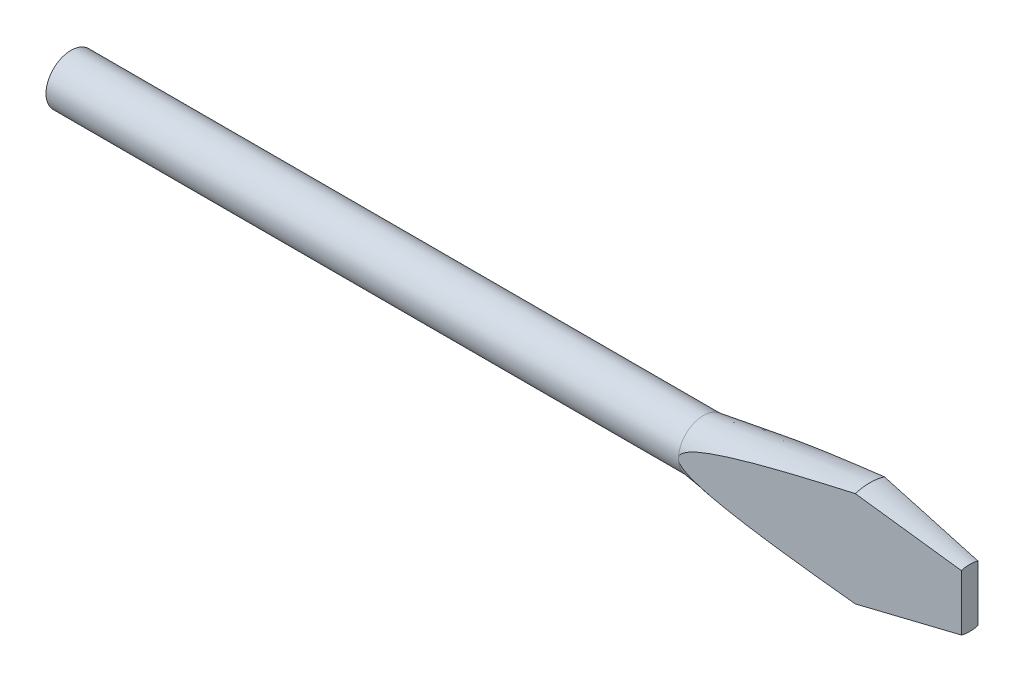
ISO-10303-21;
HEADER;
FILE_DESCRIPTION(('STEP AP214'),'2;1');
FILE_NAME('part.step','',(''),(''),'','','');
FILE_SCHEMA(('AUTOMOTIVE_DESIGN { 1 0 10303 214 1 1 1 1 }'));
ENDSEC;
DATA;
#1=APPLICATION_CONTEXT('core data for automotive mechanical design processes');
#2=APPLICATION_PROTOCOL_DEFINITION('international standard','automotive_design',2000,#1);
#3=PRODUCT_CONTEXT('',#1,'mechanical');
#4=PRODUCT('Part','Part','',(#3));
#5=PRODUCT_RELATED_PRODUCT_CATEGORY('part','',(#4));
#6=PRODUCT_DEFINITION_FORMATION('','',#4);
#7=PRODUCT_DEFINITION_CONTEXT('part definition',#1,'design');
#8=PRODUCT_DEFINITION('design','',#6,#7);
#9=PRODUCT_DEFINITION_SHAPE('','',#8);
#10=(LENGTH_UNIT() NAMED_UNIT(*) SI_UNIT(.MILLI.,.METRE.));
#11=(NAMED_UNIT(*) PLANE_ANGLE_UNIT() SI_UNIT($,.RADIAN.));
#12=(NAMED_UNIT(*) SI_UNIT($,.STERADIAN.) SOLID_ANGLE_UNIT());
#13=UNCERTAINTY_MEASURE_WITH_UNIT(LENGTH_MEASURE(1.E-05),#10,'distance_accuracy_value','');
#14=(GEOMETRIC_REPRESENTATION_CONTEXT(3) GLOBAL_UNCERTAINTY_ASSIGNED_CONTEXT((#13)) GLOBAL_UNIT_ASSIGNED_CONTEXT((#10,
#11,#12)) REPRESENTATION_CONTEXT('',''));
#15=CARTESIAN_POINT('',(0.,0.,0.));
#16=DIRECTION('',(0.,0.,1.));
#17=DIRECTION('',(1.,0.,0.));
#18=AXIS2_PLACEMENT_3D('',#15,#16,#17);
#19=CARTESIAN_POINT('',(96.,0.,0.));
#20=DIRECTION('',(1.,0.,0.));
#21=DIRECTION('',(0.,0.,-1.));
#22=AXIS2_PLACEMENT_3D('',#19,#20,#21);
#23=CONICAL_SURFACE('',#22,6.00000000000001,0.148889947609498);
#24=CARTESIAN_POINT('',(96.0002,5.73915531683399,1.7499875));
#25=CARTESIAN_POINT('',(95.5726499864452,5.66395600184694,1.77670937584718));
#26=CARTESIAN_POINT('',(95.1451987285646,5.58819220301967,1.80342507946472));
#27=CARTESIAN_POINT('',(94.2905240343786,5.43537319976455,1.85684224785134));
#28=CARTESIAN_POINT('',(93.8633005992586,5.35831798868393,1.88354371254634));
#29=CARTESIAN_POINT('',(92.5819083567461,5.12495166818705,1.96363072770337));
#30=CARTESIAN_POINT('',(91.7281335000303,4.96646016337192,2.01699165624811));
#31=CARTESIAN_POINT('',(90.019979848679,4.64146537301027,2.12375125945756));
#32=CARTESIAN_POINT('',(89.1656044854042,4.47494384895681,2.17714971966224));
#33=CARTESIAN_POINT('',(87.8856595668706,4.21721361058394,2.25714627707059));
#34=CARTESIAN_POINT('',(87.4592926054404,4.12998137074823,2.28379421215998));
#35=CARTESIAN_POINT('',(86.6072250559407,3.95231391396148,2.33704843400371));
#36=CARTESIAN_POINT('',(86.1815244633616,3.86187871878447,2.3636547210399));
#37=CARTESIAN_POINT('',(85.3312138352515,3.67715280873303,2.41679913529678));
#38=CARTESIAN_POINT('',(84.9066033099843,3.58286436326236,2.44333729312598));
#39=CARTESIAN_POINT('',(84.0584687809175,3.38939992425362,2.49634570119266));
#40=CARTESIAN_POINT('',(83.6349448230058,3.29022372775725,2.52281594856214));
#41=CARTESIAN_POINT('',(82.7896523378295,3.0856296102126,2.57564672888565));
#42=CARTESIAN_POINT('',(82.3678829429874,2.98021530209393,2.60200731606329));
#43=CARTESIAN_POINT('',(81.5265366338004,2.7609833456918,2.65459146038747));
#44=CARTESIAN_POINT('',(81.1069595251366,2.6471664562026,2.68081502967896));
#45=CARTESIAN_POINT('',(80.4071377845036,2.44647984326731,2.72455388846852));
#46=CARTESIAN_POINT('',(80.1259604528363,2.3628856653321,2.74212747169773));
#47=CARTESIAN_POINT('',(79.5658035182563,2.18838498181537,2.77713728010898));
#48=CARTESIAN_POINT('',(79.2868241923529,2.09747757025181,2.79457348797794));
#49=CARTESIAN_POINT('',(78.8218721534036,1.93636200836302,2.82363299041227));
#50=CARTESIAN_POINT('',(78.6349406666478,1.86894212685137,2.83531620833451));
#51=CARTESIAN_POINT('',(78.2634966175948,1.7278851236311,2.85853146140032));
#52=CARTESIAN_POINT('',(78.0789829462789,1.65425097650611,2.87006356585756));
#53=CARTESIAN_POINT('',(77.7692838551867,1.52206073077131,2.88941975905083));
#54=CARTESIAN_POINT('',(77.6431521485968,1.46574692133821,2.89730299071269));
#55=CARTESIAN_POINT('',(77.3933332707296,1.34752106226873,2.9129166705794));
#56=CARTESIAN_POINT('',(77.2696490920777,1.2856026199415,2.92064693174514));
#57=CARTESIAN_POINT('',(77.0267142840414,1.15443353979788,2.93583035724741));
#58=CARTESIAN_POINT('',(76.9074482122798,1.08521251318701,2.94328448673251));
#59=CARTESIAN_POINT('',(76.7339240635911,0.973178626859508,2.95412974602555));
#60=CARTESIAN_POINT('',(76.6770192579268,0.934499081121033,2.95768629637957));
#61=CARTESIAN_POINT('',(76.5657102745783,0.853705624728018,2.96464310783886));
#62=CARTESIAN_POINT('',(76.5113045369663,0.811593903283039,2.9680434664396));
#63=CARTESIAN_POINT('',(76.4109105801654,0.72706727244706,2.97431808873966));
#64=CARTESIAN_POINT('',(76.3646075046718,0.685031882048725,2.97721203095801));
#65=CARTESIAN_POINT('',(76.2763771477047,0.596432252281046,2.98272642826845));
#66=CARTESIAN_POINT('',(76.2344516319525,0.549866199953424,2.98534677300297));
#67=CARTESIAN_POINT('',(76.1638427175753,0.45942401347692,2.98975983015154));
#68=CARTESIAN_POINT('',(76.1341161979311,0.416380117894299,2.9916177376293));
#69=CARTESIAN_POINT('',(76.0817558589671,0.326142818282468,2.99489025881455));
#70=CARTESIAN_POINT('',(76.0591029434721,0.278961034526327,2.99630606603299));
#71=CARTESIAN_POINT('',(76.0287140728707,0.194604229642632,2.99820537044558));
#72=CARTESIAN_POINT('',(76.0185798334005,0.158308409565959,2.99883876041247));
#73=CARTESIAN_POINT('',(76.0045422133693,0.0845314040429726,2.99971611166441));
#74=CARTESIAN_POINT('',(76.0006312023623,0.0470517277746489,2.99996054985235));
#75=CARTESIAN_POINT('',(75.9995096958247,-0.0280966250484533,3.00003064401095));
#76=CARTESIAN_POINT('',(76.0023143668073,-0.0657655373225097,2.99985535207454));
#77=CARTESIAN_POINT('',(76.0142997316137,-0.140076870201679,2.99910626677414));
#78=CARTESIAN_POINT('',(76.0234878180765,-0.176718049349556,2.99853201137021));
#79=CARTESIAN_POINT('',(76.0511279458859,-0.259755019962619,2.99680450338213));
#80=CARTESIAN_POINT('',(76.0716181053519,-0.305460096964524,2.9955238684155));
#81=CARTESIAN_POINT('',(76.1194671645362,-0.393071508670082,2.99253330221648));
#82=CARTESIAN_POINT('',(76.1468420011463,-0.434968718132925,2.99082237492835));
#83=CARTESIAN_POINT('',(76.2308440864035,-0.548326904047211,2.98557224459977));
#84=CARTESIAN_POINT('',(76.2929683259939,-0.615651134591144,2.98168947962538));
#85=CARTESIAN_POINT('',(76.3922617223705,-0.709891572697012,2.97548364235184));
#86=CARTESIAN_POINT('',(76.4264549871577,-0.740236849569235,2.97334656330264));
#87=CARTESIAN_POINT('',(76.4964507424118,-0.79899898280661,2.96897182859926));
#88=CARTESIAN_POINT('',(76.5322524275458,-0.827416786752987,2.96673422327838));
#89=CARTESIAN_POINT('',(76.6465227232719,-0.91404425240467,2.9595923297955));
#90=CARTESIAN_POINT('',(76.7271721633252,-0.969346316998965,2.95455173979217));
#91=CARTESIAN_POINT('',(76.8919404364799,-1.07454240034944,2.94425372272));
#92=CARTESIAN_POINT('',(76.976062560228,-1.12443111923898,2.93899608998575));
#93=CARTESIAN_POINT('',(77.1468690560182,-1.2201956458567,2.92832068399886));
#94=CARTESIAN_POINT('',(77.2335603878113,-1.26605890270873,2.92290247576179));
#95=CARTESIAN_POINT('',(77.408604494444,-1.3544990689602,2.91196221909725));
#96=CARTESIAN_POINT('',(77.4969576273404,-1.39707525979243,2.90644014829122));
#97=CARTESIAN_POINT('',(77.7652954457971,-1.52153396282849,2.88966903463768));
#98=CARTESIAN_POINT('',(77.9471427155521,-1.59938497219916,2.87830358027799));
#99=CARTESIAN_POINT('',(78.2219023740701,-1.71052769479077,2.86113110162061));
#100=CARTESIAN_POINT('',(78.3137282495272,-1.74660327765731,2.85539198440454));
#101=CARTESIAN_POINT('',(78.4979891948311,-1.81715507612519,2.84387567532305));
#102=CARTESIAN_POINT('',(78.5904242395672,-1.85163135718625,2.83809848502705));
#103=CARTESIAN_POINT('',(78.8650697321673,-1.95176495296288,2.82093314173954));
#104=CARTESIAN_POINT('',(79.0479889859014,-2.01546798574804,2.80950068838116));
#105=CARTESIAN_POINT('',(79.4152004881255,-2.13878844706536,2.78654996949216));
#106=CARTESIAN_POINT('',(79.5994928565958,-2.19840551381847,2.77503169646276));
#107=CARTESIAN_POINT('',(79.9691529686513,-2.31437396895296,2.75192793945929));
#108=CARTESIAN_POINT('',(80.1545210055809,-2.37072441554196,2.74034243715119));
#109=CARTESIAN_POINT('',(80.5260554835113,-2.48072422260111,2.71712153228054));
#110=CARTESIAN_POINT('',(80.7122219450877,-2.53437351300235,2.70548612843202));
#111=CARTESIAN_POINT('',(81.2723101398846,-2.69213137866171,2.67048061625721));
#112=CARTESIAN_POINT('',(81.6471820551321,-2.79285333142643,2.64705112155424));
#113=CARTESIAN_POINT('',(82.3985506606079,-2.98767999779727,2.600090583712));
#114=CARTESIAN_POINT('',(82.7750470750032,-3.08178579123681,2.5765595578123));
#115=CARTESIAN_POINT('',(83.5271214588481,-3.26438779545831,2.52955490882199));
#116=CARTESIAN_POINT('',(83.9026924696457,-3.35291287140362,2.50608172064714));
#117=CARTESIAN_POINT('',(84.6547626031726,-3.52596598586649,2.45907733730171));
#118=CARTESIAN_POINT('',(85.0312617621282,-3.6104938656868,2.43554613986699));
#119=CARTESIAN_POINT('',(85.7846632666543,-3.77621867302195,2.3884585458341));
#120=CARTESIAN_POINT('',(86.1615650257566,-3.85741828350884,2.36490218589021));
#121=CARTESIAN_POINT('',(86.9159411464435,-4.01710542669527,2.31775367834728));
#122=CARTESIAN_POINT('',(87.2934155111964,-4.09559294433107,2.29416153055022));
#123=CARTESIAN_POINT('',(88.3622225398438,-4.31446470246228,2.22736109125976));
#124=CARTESIAN_POINT('',(89.0541012611445,-4.45217192627195,2.18411867117847));
#125=CARTESIAN_POINT('',(90.4391554801988,-4.72183662592933,2.09755278248758));
#126=CARTESIAN_POINT('',(91.1323312700355,-4.85379258700501,2.05422929562278));
#127=CARTESIAN_POINT('',(92.5210140480984,-5.11344103370427,1.96743662199385));
#128=CARTESIAN_POINT('',(93.2165228475955,-5.24112376831375,1.92396732202528));
#129=CARTESIAN_POINT('',(94.608005664441,-5.49273424440889,1.83699964597244));
#130=CARTESIAN_POINT('',(95.303979484096,-5.61666308220133,1.793501282244));
#131=CARTESIAN_POINT('',(96.0002,-5.73915531683399,1.7499875));
#132=B_SPLINE_CURVE_WITH_KNOTS('',3,(#24,#25,#26,#27,#28,#29,#30,#31,#32,#33,#34,#35,#36,#37,
#38,#39,#40,#41,#42,#43,#44,#45,#46,#47,#48,#49,#50,#51,#52,#53,#54,#55,#56,#57,#58,#59,#60,#61,
#62,#63,#64,#65,#66,#67,#68,#69,#70,#71,#72,#73,#74,#75,#76,#77,#78,#79,#80,#81,#82,#83,#84,#85,
#86,#87,#88,#89,#90,#91,#92,#93,#94,#95,#96,#97,#98,#99,#100,#101,#102,#103,#104,#105,#106,#107,
#108,#109,#110,#111,#112,#113,#114,#115,#116,#117,#118,#119,#120,#121,#122,#123,#124,#125,#126,
#127,#128,#129,#130,#131),.UNSPECIFIED.,.F.,.F.,(4,2,2,2,2,2,2,2,2,2,2,2,2,2,2,2,2,2,2,2,2,2,2,
2,2,2,2,2,2,2,2,2,2,2,2,2,2,2,2,2,2,2,2,2,2,2,2,2,2,2,2,2,2,4),(0.,1.30480309700493,
2.60961291782616,5.21958617375214,7.83579570800606,9.14382881698877,10.4518530355277,
11.7591176818992,13.0664366567582,14.3730057440394,15.6794569857201,16.560993285378,
17.4426389606708,18.0397485388532,18.6365739022333,19.0515421216089,19.4669897694782,
19.8808132452841,20.0874146908788,20.2938853721059,20.4814844272004,20.6691588618109,
20.8257442211872,20.9819031270959,21.0945089102319,21.2069765180959,21.319698359208,
21.4325509616643,21.5820062092499,21.7318106577102,22.0052437671489,22.1425333848363,
22.2797550117329,22.5731679806603,22.8668656680802,23.1614487484508,23.4560960447131,
24.0502122915525,24.3466823999598,24.6431403630655,25.2251663035284,25.8072437112532,
26.3894881102989,26.9717476051897,28.1382741975795,29.3046099552705,30.4643109542367,
31.6240579572255,32.7828509057353,33.941650289479,36.061935301918,38.1827754230579,
40.3081641870455,42.4329261372792),.UNSPECIFIED.);
#133=CARTESIAN_POINT('',(96.,5.7391201416245,1.75));
#134=VERTEX_POINT('',#133);
#135=CARTESIAN_POINT('',(76.,0.,2.99999999999999));
#136=VERTEX_POINT('',#135);
#137=EDGE_CURVE('E96',#134,#136,#132,.T.);
#138=ORIENTED_EDGE('',*,*,#137,.F.);
#139=CARTESIAN_POINT('',(96.,0.,0.));
#140=DIRECTION('',(-1.,0.,0.));
#141=DIRECTION('',(0.,0.,1.));
#142=AXIS2_PLACEMENT_3D('',#139,#140,#141);
#143=CIRCLE('',#142,6.00000000000001);
#144=CARTESIAN_POINT('',(96.,5.7391201416245,-1.75));
#145=VERTEX_POINT('',#144);
#146=EDGE_CURVE('E94',#134,#145,#143,.T.);
#147=ORIENTED_EDGE('',*,*,#146,.T.);
#148=CARTESIAN_POINT('',(96.0002,5.73915531683399,-1.7499875));
#149=CARTESIAN_POINT('',(95.5726499864452,5.66395600184694,-1.77670937584718));
#150=CARTESIAN_POINT('',(95.1451987285646,5.58819220301967,-1.80342507946472));
#151=CARTESIAN_POINT('',(94.2905240343786,5.43537319976455,-1.85684224785134));
#152=CARTESIAN_POINT('',(93.8633005992586,5.35831798868393,-1.88354371254634));
#153=CARTESIAN_POINT('',(92.5819083567461,5.12495166818705,-1.96363072770337));
#154=CARTESIAN_POINT('',(91.7281335000303,4.96646016337192,-2.01699165624811));
#155=CARTESIAN_POINT('',(90.019979848679,4.64146537301027,-2.12375125945756));
#156=CARTESIAN_POINT('',(89.1656044854042,4.47494384895681,-2.17714971966224));
#157=CARTESIAN_POINT('',(87.8856595668706,4.21721361058394,-2.25714627707059));
#158=CARTESIAN_POINT('',(87.4592926054404,4.12998137074823,-2.28379421215998));
#159=CARTESIAN_POINT('',(86.6072250559407,3.95231391396148,-2.33704843400371));
#160=CARTESIAN_POINT('',(86.1815244633616,3.86187871878447,-2.3636547210399));
#161=CARTESIAN_POINT('',(85.3312138352515,3.67715280873303,-2.41679913529678));
#162=CARTESIAN_POINT('',(84.9066033099843,3.58286436326236,-2.44333729312598));
#163=CARTESIAN_POINT('',(84.0584687809175,3.38939992425362,-2.49634570119266));
#164=CARTESIAN_POINT('',(83.6349448230058,3.29022372775725,-2.52281594856214));
#165=CARTESIAN_POINT('',(82.7896523378295,3.0856296102126,-2.57564672888565));
#166=CARTESIAN_POINT('',(82.3678829429874,2.98021530209393,-2.60200731606329));
#167=CARTESIAN_POINT('',(81.5265366338004,2.7609833456918,-2.65459146038747));
#168=CARTESIAN_POINT('',(81.1069595251366,2.6471664562026,-2.68081502967896));
#169=CARTESIAN_POINT('',(80.4071377845036,2.44647984326731,-2.72455388846852));
#170=CARTESIAN_POINT('',(80.1259604528363,2.3628856653321,-2.74212747169773));
#171=CARTESIAN_POINT('',(79.5658035182563,2.18838498181537,-2.77713728010898));
#172=CARTESIAN_POINT('',(79.2868241923529,2.09747757025181,-2.79457348797794));
#173=CARTESIAN_POINT('',(78.8218721534036,1.93636200836302,-2.82363299041227));
#174=CARTESIAN_POINT('',(78.6349406666478,1.86894212685137,-2.83531620833451));
#175=CARTESIAN_POINT('',(78.2634966175948,1.7278851236311,-2.85853146140032));
#176=CARTESIAN_POINT('',(78.0789829462789,1.65425097650611,-2.87006356585756));
#177=CARTESIAN_POINT('',(77.7692838551867,1.52206073077131,-2.88941975905083));
#178=CARTESIAN_POINT('',(77.6431521485968,1.46574692133821,-2.89730299071269));
#179=CARTESIAN_POINT('',(77.3933332707296,1.34752106226873,-2.9129166705794));
#180=CARTESIAN_POINT('',(77.2696490920777,1.2856026199415,-2.92064693174514));
#181=CARTESIAN_POINT('',(77.0267142840414,1.15443353979788,-2.93583035724741));
#182=CARTESIAN_POINT('',(76.9074482122798,1.08521251318701,-2.94328448673251));
#183=CARTESIAN_POINT('',(76.7339240635911,0.973178626859508,-2.95412974602555));
#184=CARTESIAN_POINT('',(76.6770192579268,0.934499081121033,-2.95768629637957));
#185=CARTESIAN_POINT('',(76.5657102745783,0.853705624728018,-2.96464310783886));
#186=CARTESIAN_POINT('',(76.5113045369663,0.811593903283039,-2.9680434664396));
#187=CARTESIAN_POINT('',(76.4109105801654,0.72706727244706,-2.97431808873966));
#188=CARTESIAN_POINT('',(76.3646075046718,0.685031882048725,-2.97721203095801));
#189=CARTESIAN_POINT('',(76.2763771477047,0.596432252281046,-2.98272642826845));
#190=CARTESIAN_POINT('',(76.2344516319525,0.549866199953424,-2.98534677300297));
#191=CARTESIAN_POINT('',(76.1638427175753,0.45942401347692,-2.98975983015154));
#192=CARTESIAN_POINT('',(76.1341161979311,0.416380117894299,-2.9916177376293));
#193=CARTESIAN_POINT('',(76.0817558589671,0.326142818282468,-2.99489025881455));
#194=CARTESIAN_POINT('',(76.0591029434721,0.278961034526327,-2.99630606603299));
#195=CARTESIAN_POINT('',(76.0287140728707,0.194604229642632,-2.99820537044558));
#196=CARTESIAN_POINT('',(76.0185798334005,0.158308409565959,-2.99883876041247));
#197=CARTESIAN_POINT('',(76.0045422133693,0.0845314040429726,-2.99971611166441));
#198=CARTESIAN_POINT('',(76.0006312023623,0.0470517277746489,-2.99996054985235));
#199=CARTESIAN_POINT('',(75.9995096958247,-0.0280966250484533,-3.00003064401095));
#200=CARTESIAN_POINT('',(76.0023143668073,-0.0657655373225097,-2.99985535207454));
#201=CARTESIAN_POINT('',(76.0142997316137,-0.140076870201679,-2.99910626677414));
#202=CARTESIAN_POINT('',(76.0234878180765,-0.176718049349556,-2.99853201137021));
#203=CARTESIAN_POINT('',(76.0511279458859,-0.259755019962619,-2.99680450338213));
#204=CARTESIAN_POINT('',(76.0716181053519,-0.305460096964524,-2.9955238684155));
#205=CARTESIAN_POINT('',(76.1194671645362,-0.393071508670082,-2.99253330221648));
#206=CARTESIAN_POINT('',(76.1468420011463,-0.434968718132925,-2.99082237492835));
#207=CARTESIAN_POINT('',(76.2308440864035,-0.548326904047211,-2.98557224459977));
#208=CARTESIAN_POINT('',(76.2929683259939,-0.615651134591144,-2.98168947962538));
#209=CARTESIAN_POINT('',(76.3922617223705,-0.709891572697012,-2.97548364235184));
#210=CARTESIAN_POINT('',(76.4264549871577,-0.740236849569235,-2.97334656330264));
#211=CARTESIAN_POINT('',(76.4964507424118,-0.79899898280661,-2.96897182859926));
#212=CARTESIAN_POINT('',(76.5322524275458,-0.827416786752987,-2.96673422327838));
#213=CARTESIAN_POINT('',(76.6465227232719,-0.91404425240467,-2.9595923297955));
#214=CARTESIAN_POINT('',(76.7271721633252,-0.969346316998965,-2.95455173979217));
#215=CARTESIAN_POINT('',(76.8919404364799,-1.07454240034944,-2.94425372272));
#216=CARTESIAN_POINT('',(76.976062560228,-1.12443111923898,-2.93899608998575));
#217=CARTESIAN_POINT('',(77.1468690560182,-1.2201956458567,-2.92832068399886));
#218=CARTESIAN_POINT('',(77.2335603878113,-1.26605890270873,-2.92290247576179));
#219=CARTESIAN_POINT('',(77.408604494444,-1.3544990689602,-2.91196221909725));
#220=CARTESIAN_POINT('',(77.4969576273404,-1.39707525979243,-2.90644014829122));
#221=CARTESIAN_POINT('',(77.7652954457971,-1.52153396282849,-2.88966903463768));
#222=CARTESIAN_POINT('',(77.9471427155521,-1.59938497219916,-2.87830358027799));
#223=CARTESIAN_POINT('',(78.2219023740701,-1.71052769479077,-2.86113110162061));
#224=CARTESIAN_POINT('',(78.3137282495272,-1.74660327765731,-2.85539198440454));
#225=CARTESIAN_POINT('',(78.4979891948311,-1.81715507612519,-2.84387567532305));
#226=CARTESIAN_POINT('',(78.5904242395672,-1.85163135718625,-2.83809848502705));
#227=CARTESIAN_POINT('',(78.8650697321673,-1.95176495296288,-2.82093314173954));
#228=CARTESIAN_POINT('',(79.0479889859014,-2.01546798574804,-2.80950068838116));
#229=CARTESIAN_POINT('',(79.4152004881255,-2.13878844706536,-2.78654996949216));
#230=CARTESIAN_POINT('',(79.5994928565958,-2.19840551381847,-2.77503169646276));
#231=CARTESIAN_POINT('',(79.9691529686513,-2.31437396895296,-2.75192793945929));
#232=CARTESIAN_POINT('',(80.1545210055809,-2.37072441554196,-2.74034243715119));
#233=CARTESIAN_POINT('',(80.5260554835113,-2.48072422260111,-2.71712153228054));
#234=CARTESIAN_POINT('',(80.7122219450877,-2.53437351300235,-2.70548612843202));
#235=CARTESIAN_POINT('',(81.2723101398846,-2.69213137866171,-2.67048061625721));
#236=CARTESIAN_POINT('',(81.6471820551321,-2.79285333142643,-2.64705112155424));
#237=CARTESIAN_POINT('',(82.3985506606079,-2.98767999779727,-2.600090583712));
#238=CARTESIAN_POINT('',(82.7750470750032,-3.08178579123681,-2.5765595578123));
#239=CARTESIAN_POINT('',(83.5271214588481,-3.26438779545831,-2.52955490882199));
#240=CARTESIAN_POINT('',(83.9026924696457,-3.35291287140362,-2.50608172064714));
#241=CARTESIAN_POINT('',(84.6547626031726,-3.52596598586649,-2.45907733730171));
#242=CARTESIAN_POINT('',(85.0312617621282,-3.6104938656868,-2.43554613986699));
#243=CARTESIAN_POINT('',(85.7846632666543,-3.77621867302195,-2.3884585458341));
#244=CARTESIAN_POINT('',(86.1615650257566,-3.85741828350884,-2.36490218589021));
#245=CARTESIAN_POINT('',(86.9159411464435,-4.01710542669527,-2.31775367834728));
#246=CARTESIAN_POINT('',(87.2934155111964,-4.09559294433107,-2.29416153055022));
#247=CARTESIAN_POINT('',(88.3622225398438,-4.31446470246228,-2.22736109125976));
#248=CARTESIAN_POINT('',(89.0541012611445,-4.45217192627195,-2.18411867117847));
#249=CARTESIAN_POINT('',(90.4391554801988,-4.72183662592933,-2.09755278248758));
#250=CARTESIAN_POINT('',(91.1323312700355,-4.85379258700501,-2.05422929562278));
#251=CARTESIAN_POINT('',(92.5210140480984,-5.11344103370427,-1.96743662199385));
#252=CARTESIAN_POINT('',(93.2165228475955,-5.24112376831375,-1.92396732202528));
#253=CARTESIAN_POINT('',(94.608005664441,-5.49273424440889,-1.83699964597244));
#254=CARTESIAN_POINT('',(95.303979484096,-5.61666308220133,-1.793501282244));
#255=CARTESIAN_POINT('',(96.0002,-5.73915531683399,-1.7499875));
#256=B_SPLINE_CURVE_WITH_KNOTS('',3,(#148,#149,#150,#151,#152,#153,#154,#155,#156,#157,#158,
#159,#160,#161,#162,#163,#164,#165,#166,#167,#168,#169,#170,#171,#172,#173,#174,#175,#176,#177,
#178,#179,#180,#181,#182,#183,#184,#185,#186,#187,#188,#189,#190,#191,#192,#193,#194,#195,#196,
#197,#198,#199,#200,#201,#202,#203,#204,#205,#206,#207,#208,#209,#210,#211,#212,#213,#214,#215,
#216,#217,#218,#219,#220,#221,#222,#223,#224,#225,#226,#227,#228,#229,#230,#231,#232,#233,#234,
#235,#236,#237,#238,#239,#240,#241,#242,#243,#244,#245,#246,#247,#248,#249,#250,#251,#252,#253,
#254,#255),.UNSPECIFIED.,.F.,.F.,(4,2,2,2,2,2,2,2,2,2,2,2,2,2,2,2,2,2,2,2,2,2,2,2,2,2,2,2,2,2,2,
2,2,2,2,2,2,2,2,2,2,2,2,2,2,2,2,2,2,2,2,2,2,4),(0.,1.30480309700493,2.60961291782616,
5.21958617375214,7.83579570800606,9.14382881698877,10.4518530355277,11.7591176818992,
13.0664366567582,14.3730057440394,15.6794569857201,16.560993285378,17.4426389606708,
18.0397485388532,18.6365739022333,19.0515421216089,19.4669897694782,19.8808132452841,
20.0874146908788,20.2938853721059,20.4814844272004,20.6691588618109,20.8257442211872,
20.9819031270959,21.0945089102319,21.2069765180959,21.319698359208,21.4325509616643,
21.5820062092499,21.7318106577102,22.0052437671489,22.1425333848363,22.2797550117329,
22.5731679806603,22.8668656680802,23.1614487484508,23.4560960447131,24.0502122915525,
24.3466823999598,24.6431403630655,25.2251663035284,25.8072437112532,26.3894881102989,
26.9717476051897,28.1382741975795,29.3046099552705,30.4643109542367,31.6240579572255,
32.7828509057353,33.941650289479,36.061935301918,38.1827754230579,40.3081641870455,
42.4329261372792),.UNSPECIFIED.);
#257=CARTESIAN_POINT('',(76.,0.,-2.99999999999999));
#258=VERTEX_POINT('',#257);
#259=EDGE_CURVE('E103',#145,#258,#256,.T.);
#260=ORIENTED_EDGE('',*,*,#259,.T.);
#261=CARTESIAN_POINT('',(76.,0.,0.));
#262=DIRECTION('',(-1.,0.,0.));
#263=DIRECTION('',(0.,0.,1.));
#264=AXIS2_PLACEMENT_3D('',#261,#262,#263);
#265=CIRCLE('',#264,2.99999999999999);
#266=EDGE_CURVE('E116',#136,#258,#265,.T.);
#267=ORIENTED_EDGE('',*,*,#266,.F.);
#268=EDGE_LOOP('',(#138,#147,#260,#267));
#269=FACE_BOUND('',#268,.T.);
#270=ADVANCED_FACE('F41',(#269),#23,.T.);
#271=CARTESIAN_POINT('',(96.,-5.7391201416245,1.75));
#272=VERTEX_POINT('',#271);
#273=EDGE_CURVE('E139',#136,#272,#132,.T.);
#274=ORIENTED_EDGE('',*,*,#273,.F.);
#275=EDGE_CURVE('E120',#258,#136,#265,.T.);
#276=ORIENTED_EDGE('',*,*,#275,.F.);
#277=CARTESIAN_POINT('',(96.,-5.7391201416245,-1.75));
#278=VERTEX_POINT('',#277);
#279=EDGE_CURVE('E137',#258,#278,#256,.T.);
#280=ORIENTED_EDGE('',*,*,#279,.T.);
#281=EDGE_CURVE('E114',#278,#272,#143,.T.);
#282=ORIENTED_EDGE('',*,*,#281,.T.);
#283=EDGE_LOOP('',(#274,#276,#280,#282));
#284=FACE_BOUND('',#283,.T.);
#285=ADVANCED_FACE('F134',(#284),#23,.T.);
#286=CARTESIAN_POINT('',(108.,0.,0.));
#287=DIRECTION('',(-1.,0.,0.));
#288=DIRECTION('',(0.,0.,1.));
#289=AXIS2_PLACEMENT_3D('',#286,#287,#288);
#290=CONICAL_SURFACE('',#289,3.5,0.205395389189769);
#291=CARTESIAN_POINT('',(108.0002,3.35406221393002,0.999987500000007));
#292=CARTESIAN_POINT('',(106.102909473185,3.73116588658497,1.11856815792595));
#293=CARTESIAN_POINT('',(104.205617653798,4.10826303038711,1.23714889663762));
#294=CARTESIAN_POINT('',(100.205484615702,4.90329708058614,1.48715721151863));
#295=CARTESIAN_POINT('',(98.1026431017553,5.32123249572359,1.6185848061403));
#296=CARTESIAN_POINT('',(95.9998,5.73915989074881,1.7500125));
#297=B_SPLINE_CURVE_WITH_KNOTS('',3,(#291,#292,#293,#294,#295,#296),.UNSPECIFIED.,.F.,.F.,(4,2,
4),(0.,5.81410518122257,12.258092371595),.UNSPECIFIED.);
#298=CARTESIAN_POINT('',(108.,3.35410196624968,1.));
#299=VERTEX_POINT('',#298);
#300=EDGE_CURVE('E87',#299,#134,#297,.T.);
#301=ORIENTED_EDGE('',*,*,#300,.F.);
#302=CARTESIAN_POINT('',(108.,0.,0.));
#303=DIRECTION('',(-1.,0.,0.));
#304=DIRECTION('',(0.,0.,1.));
#305=AXIS2_PLACEMENT_3D('',#302,#303,#304);
#306=CIRCLE('',#305,3.5);
#307=CARTESIAN_POINT('',(108.,3.35410196624968,-1.00000000000001));
#308=VERTEX_POINT('',#307);
#309=EDGE_CURVE('E62',#299,#308,#306,.T.);
#310=ORIENTED_EDGE('',*,*,#309,.T.);
#311=CARTESIAN_POINT('',(108.0002,3.35406221393002,-0.999987500000007));
#312=CARTESIAN_POINT('',(106.102909473185,3.73116588658497,-1.11856815792595));
#313=CARTESIAN_POINT('',(104.205617653798,4.10826303038711,-1.23714889663762));
#314=CARTESIAN_POINT('',(100.205484615702,4.90329708058614,-1.48715721151863));
#315=CARTESIAN_POINT('',(98.1026431017553,5.32123249572359,-1.6185848061403));
#316=CARTESIAN_POINT('',(95.9998,5.73915989074881,-1.7500125));
#317=B_SPLINE_CURVE_WITH_KNOTS('',3,(#311,#312,#313,#314,#315,#316),.UNSPECIFIED.,.F.,.F.,(4,2,
4),(0.,5.81410518122257,12.258092371595),.UNSPECIFIED.);
#318=EDGE_CURVE('E101',#308,#145,#317,.T.);
#319=ORIENTED_EDGE('',*,*,#318,.T.);
#320=ORIENTED_EDGE('',*,*,#146,.F.);
#321=EDGE_LOOP('',(#301,#310,#319,#320));
#322=FACE_BOUND('',#321,.T.);
#323=ADVANCED_FACE('F91',(#322),#290,.T.);
#324=CARTESIAN_POINT('',(95.9998,-5.73915989074881,1.7500125));
#325=CARTESIAN_POINT('',(99.2523695402323,-5.09273571894703,1.54672690373549));
#326=CARTESIAN_POINT('',(102.504934596358,-4.44628889795995,1.34344158772766));
#327=CARTESIAN_POINT('',(106.505063682463,-3.65123488631053,1.09343351984605));
#328=CARTESIAN_POINT('',(107.252631959671,-3.50264914835802,1.04671050252055));
#329=CARTESIAN_POINT('',(108.0002,-3.35406221393002,0.999987500000007));
#330=B_SPLINE_CURVE_WITH_KNOTS('',3,(#324,#325,#326,#327,#328,#329),.UNSPECIFIED.,.F.,.F.,(4,2,
4),(0.,9.96722532641675,12.2580923715829),.UNSPECIFIED.);
#331=CARTESIAN_POINT('',(108.,-3.35410196624968,1.00000000000001));
#332=VERTEX_POINT('',#331);
#333=EDGE_CURVE('E54',#272,#332,#330,.T.);
#334=ORIENTED_EDGE('',*,*,#333,.F.);
#335=ORIENTED_EDGE('',*,*,#281,.F.);
#336=CARTESIAN_POINT('',(95.9998,-5.73915989074881,-1.7500125));
#337=CARTESIAN_POINT('',(99.2523695402323,-5.09273571894703,-1.54672690373549));
#338=CARTESIAN_POINT('',(102.504934596358,-4.44628889795995,-1.34344158772766));
#339=CARTESIAN_POINT('',(106.505063682463,-3.65123488631053,-1.09343351984605));
#340=CARTESIAN_POINT('',(107.252631959671,-3.50264914835802,-1.04671050252055));
#341=CARTESIAN_POINT('',(108.0002,-3.35406221393002,-0.999987500000007));
#342=B_SPLINE_CURVE_WITH_KNOTS('',3,(#336,#337,#338,#339,#340,#341),.UNSPECIFIED.,.F.,.F.,(4,2,
4),(0.,9.96722532641675,12.2580923715829),.UNSPECIFIED.);
#343=CARTESIAN_POINT('',(108.,-3.35410196624968,-1.));
#344=VERTEX_POINT('',#343);
#345=EDGE_CURVE('E92',#278,#344,#342,.T.);
#346=ORIENTED_EDGE('',*,*,#345,.T.);
#347=EDGE_CURVE('E99',#344,#332,#306,.T.);
#348=ORIENTED_EDGE('',*,*,#347,.T.);
#349=EDGE_LOOP('',(#334,#335,#346,#348));
#350=FACE_BOUND('',#349,.T.);
#351=ADVANCED_FACE('F162',(#350),#290,.T.);
#352=CARTESIAN_POINT('',(108.,3.5,0.));
#353=DIRECTION('',(-1.,0.,0.));
#354=DIRECTION('',(0.,0.,1.));
#355=AXIS2_PLACEMENT_3D('',#352,#353,#354);
#356=PLANE('',#355);
#357=DIRECTION('',(0.,1.,0.));
#358=VECTOR('',#357,1.);
#359=CARTESIAN_POINT('',(108.,3.5,1.00000000000001));
#360=LINE('',#359,#358);
#361=EDGE_CURVE('E11',#332,#299,#360,.T.);
#362=ORIENTED_EDGE('',*,*,#361,.F.);
#363=ORIENTED_EDGE('',*,*,#347,.F.);
#364=DIRECTION('',(0.,1.,0.));
#365=VECTOR('',#364,1.);
#366=CARTESIAN_POINT('',(108.,3.5,-1.00000000000001));
#367=LINE('',#366,#365);
#368=EDGE_CURVE('E47',#344,#308,#367,.T.);
#369=ORIENTED_EDGE('',*,*,#368,.T.);
#370=ORIENTED_EDGE('',*,*,#309,.F.);
#371=EDGE_LOOP('',(#362,#363,#369,#370));
#372=FACE_BOUND('',#371,.T.);
#373=ADVANCED_FACE('F97',(#372),#356,.F.);
#374=CARTESIAN_POINT('',(0.,0.,0.));
#375=DIRECTION('',(1.,0.,0.));
#376=DIRECTION('',(0.,0.,-1.));
#377=AXIS2_PLACEMENT_3D('',#374,#375,#376);
#378=PLANE('',#377);
#379=CARTESIAN_POINT('',(0.,0.,0.));
#380=DIRECTION('',(-1.,0.,0.));
#381=DIRECTION('',(0.,0.,1.));
#382=AXIS2_PLACEMENT_3D('',#379,#380,#381);
#383=CIRCLE('',#382,2.99999999999999);
#384=CARTESIAN_POINT('',(0.,0.,2.99999999999999));
#385=VERTEX_POINT('',#384);
#386=EDGE_CURVE('E119',#385,#385,#383,.T.);
#387=ORIENTED_EDGE('',*,*,#386,.T.);
#388=EDGE_LOOP('',(#387));
#389=FACE_BOUND('',#388,.T.);
#390=ADVANCED_FACE('F43',(#389),#378,.F.);
#391=CARTESIAN_POINT('',(-206.404998063232,0.,0.));
#392=DIRECTION('',(-1.,0.,0.));
#393=DIRECTION('',(0.,0.,1.));
#394=AXIS2_PLACEMENT_3D('',#391,#392,#393);
#395=CYLINDRICAL_SURFACE('',#394,2.99999999999999);
#396=ORIENTED_EDGE('',*,*,#386,.F.);
#397=EDGE_LOOP('',(#396));
#398=FACE_BOUND('',#397,.T.);
#399=ORIENTED_EDGE('',*,*,#275,.T.);
#400=ORIENTED_EDGE('',*,*,#266,.T.);
#401=EDGE_LOOP('',(#399,#400));
#402=FACE_BOUND('',#401,.T.);
#403=ADVANCED_FACE('F123',(#398,#402),#395,.T.);
#404=CARTESIAN_POINT('',(108.,-10.,-1.));
#405=DIRECTION('',(-0.0623782861551802,0.,0.998052578482889));
#406=DIRECTION('',(0.998052578482889,0.,0.0623782861551802));
#407=AXIS2_PLACEMENT_3D('',#404,#405,#406);
#408=PLANE('',#407);
#409=ORIENTED_EDGE('',*,*,#368,.F.);
#410=ORIENTED_EDGE('',*,*,#345,.F.);
#411=ORIENTED_EDGE('',*,*,#279,.F.);
#412=ORIENTED_EDGE('',*,*,#259,.F.);
#413=ORIENTED_EDGE('',*,*,#318,.F.);
#414=EDGE_LOOP('',(#409,#410,#411,#412,#413));
#415=FACE_BOUND('',#414,.T.);
#416=ADVANCED_FACE('F126',(#415),#408,.F.);
#417=CARTESIAN_POINT('',(108.,-10.,1.));
#418=DIRECTION('',(0.0623782861551802,0.,0.998052578482889));
#419=DIRECTION('',(0.998052578482889,0.,-0.0623782861551802));
#420=AXIS2_PLACEMENT_3D('',#417,#418,#419);
#421=PLANE('',#420);
#422=ORIENTED_EDGE('',*,*,#300,.T.);
#423=ORIENTED_EDGE('',*,*,#137,.T.);
#424=ORIENTED_EDGE('',*,*,#273,.T.);
#425=ORIENTED_EDGE('',*,*,#333,.T.);
#426=ORIENTED_EDGE('',*,*,#361,.T.);
#427=EDGE_LOOP('',(#422,#423,#424,#425,#426));
#428=FACE_BOUND('',#427,.T.);
#429=ADVANCED_FACE('F88',(#428),#421,.T.);
#430=CLOSED_SHELL('',(#270,#285,#323,#351,#373,#390,#403,#416,#429));
#431=MANIFOLD_SOLID_BREP('B2',#430);
#432=ADVANCED_BREP_SHAPE_REPRESENTATION('',(#18,#431),#14);
#433=SHAPE_DEFINITION_REPRESENTATION(#9,#432);
ENDSEC;
END-ISO-10303-21;
